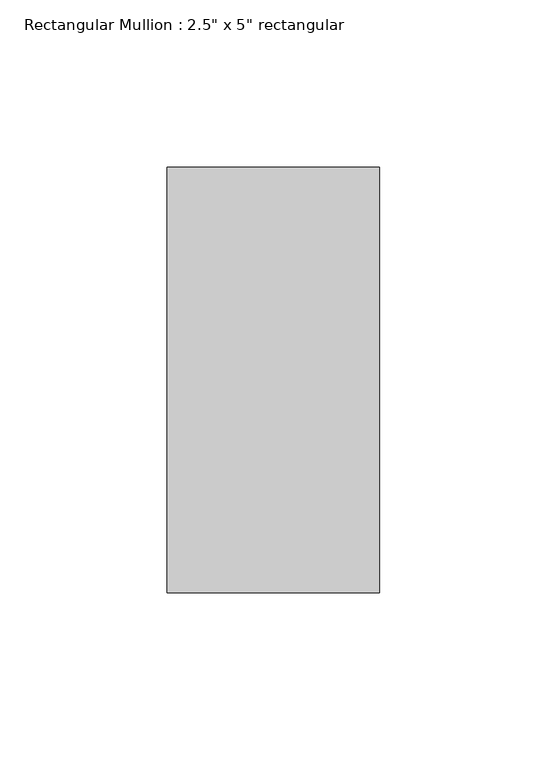
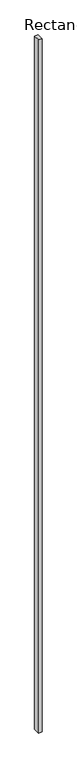
"""IFC4 building model written with IfcOpenShell, lengths in millimetres: member geometry."""

from ifc_helpers import new_model, si_unit, frame, origin, place, context, project, spatial, polyline, outline, extrude, source, transform, mapped, element, save


def member_9867d003(model_context):
    return source(origin(), model_context, "Body", "SweptSolid", [
        extrude(outline(polyline([(0.0, 63.5), (0.0, -63.5), (-63.5, -63.5), (-63.5, 63.5), (0.0, 63.5)])), frame((0.0, 0.0, -13691.4471497), z_axis=(0.0, 0.0, 1.0), x_axis=(1.0, 0.0, 0.0)), (0.0, 0.0, 1.0), 13691.4471497),
    ])


if __name__ == "__main__":
    model = new_model("IFC4")
    model_context = context("Model", 3, world=origin())
    ifc_project = project(units=[si_unit("LENGTHUNIT", "METRE", prefix="MILLI")], contexts=[model_context])
    site = spatial("IfcSite", under=ifc_project)
    building = spatial("IfcBuilding", under=site)
    placement = place(None, origin())
    member_shape = member_9867d003(model_context)
    element("IfcMember", 1, ObjectType="Rectangular Mullion : 2.5\" x 5\" rectangular", at=placement, inside=building, context=model_context, shape_type="MappedRepresentation", body=[
        mapped(member_shape, transform((0.0, 0.0, 0.0), x_axis=(1.0, 0.0, 0.0), y_axis=(0.0, 1.0, 0.0), z_axis=(0.0, 0.0, 1.0))),
    ])
    save(model, "model.ifc")

# Revit data of these elements
# Type "Rectangular Mullion : 2.5\" x 5\" rectangular"
#   built-in parameter 1007304 = 0.416667 (stored number, unit not read)
#   built-in parameter 1007301 = 0.104167 (stored number, unit not read)
#   built-in parameter 1007300 = 0.104167 (stored number, unit not read)
# Element 1 (IfcMember, "Rectangular Mullion : 2.5\" x 5\" rectangular")
#   Materials on its faces: "Aluminum"
# Materials
#   "Aluminum": class "Metal", colour RGB 247 247 247, transparency 0, Description = "Aluminum 6061", Cost = 0
